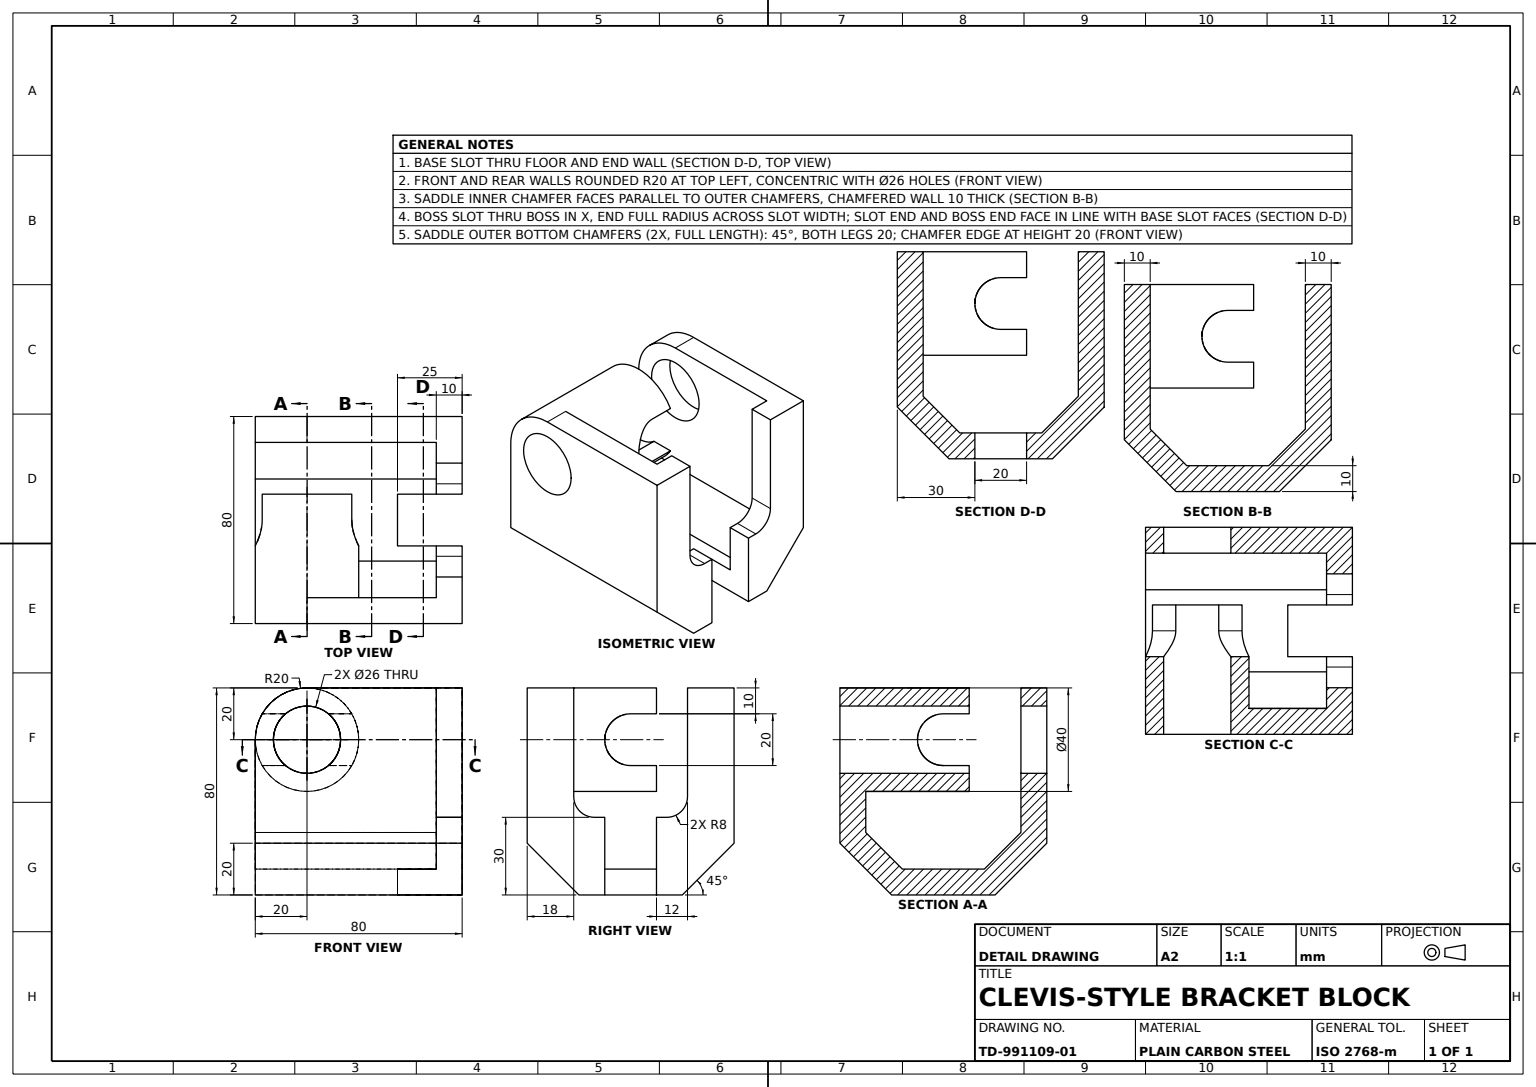
from build123d import *

# Parameters (mm, degrees)
SADDLE_BODY_DEPTH     = 40
ARM_TOP_ROUNDS_R20_R  = 20
SIDE_BOSS_DEPTH       = 10
BOSS_POCKET_SKETCH_W  = 20
BOSS_POCKET_SKETCH_H  = 10
BOSS_POCKET_CUT_DEPTH = 25
JOURNAL_BOSS_SKETCH_R = 20
JOURNAL_BOSS_DEPTH    = 40
BASE_SLOT_20X60_DEPTH = 98.979589711
JOURNAL_BORE_SKETCH_R = 13
JOURNAL_BORE_26_DEPTH = 121.0000001


with BuildPart() as part:
    # Saddle Profile Sketch → Saddle Body (new, symmetric)
    with BuildSketch(Plane(origin=(0, 0, 0), x_dir=(0, 0, -1), z_dir=(1, 0, 0))):
        Polygon((-20, 0), (20, 0), (40, 20), (40, 80), (30, 80), (30, 24.142135624), (15.857864376, 10), (-15.857864376, 10), (-30, 24.142135624), (-30, 80), (-40, 80), (-40, 20), align=None)
    extrude(amount=SADDLE_BODY_DEPTH, both=True)

    # Arm Top Rounds R20
    arm_top_rounds_r20_edges = [part.edges().sort_by_distance(p)[0] for p in [
        (-40, 80, 35),
        (-40, 80, -35),
    ]]
    fillet(arm_top_rounds_r20_edges, radius=ARM_TOP_ROUNDS_R20_R)

    # Side Boss Sketch → Side Boss (add)
    with BuildSketch(Plane(origin=(40, 0, 0), x_dir=(0, 0, -1), z_dir=(1, 0, 0))):
        with BuildLine():
            Line((-30, 80), (-22, 80))
            Line((-22, 80), (-22, 38))
            ThreePointArc((-22, 38), (-19.656854249, 32.343145751), (-14, 30))
            Line((-14, 30), (-10, 30))
            Line((-10, 30), (-10, 10))
            Line((-10, 10), (-15.857864376, 10))
            Line((-15.857864376, 10), (-30, 24.142135624))
            Line((-30, 24.142135624), (-30, 80))
        make_face()
        with BuildLine():
            Line((10, 30), (10, 10))
            Line((10, 10), (15.857864376, 10))
            Line((15.857864376, 10), (30, 24.142135624))
            Line((30, 24.142135624), (30, 80))
            Line((30, 80), (22, 80))
            Line((22, 80), (22, 38))
            ThreePointArc((22, 38), (19.656854249, 32.343145751), (14, 30))
            Line((14, 30), (10, 30))
        make_face()
    extrude(amount=-SIDE_BOSS_DEPTH)

    # Boss Pocket Sketch → Boss Pocket Cut (cut)
    with BuildSketch(Plane(origin=(40, 0, 0), x_dir=(0, 0, -1), z_dir=(1, 0, 0))):
        with Locations((0, 5)):
            Rectangle(BOSS_POCKET_SKETCH_W, BOSS_POCKET_SKETCH_H)
    extrude(amount=-BOSS_POCKET_CUT_DEPTH, mode=Mode.SUBTRACT)

    # Journal Boss Sketch → Journal Boss (add)
    with BuildSketch(Plane(origin=(0, 0, 30), x_dir=(-1, 0, 0), z_dir=(0, 0, -1))):
        with Locations(Location((20, 60, 0), (0, 0, 90))):
            Circle(JOURNAL_BOSS_SKETCH_R)
    extrude(amount=JOURNAL_BOSS_DEPTH)

    # Base Slot Sketch → Base Slot 20x60 (cut, through all)
    with BuildSketch(Plane(origin=(0, 0, 0), x_dir=(0, 0, -1), z_dir=(1, 0, 0))):
        with BuildLine():
            Line((0, 70), (14.531264235, 70))
            Line((14.531264235, 70), (14.531264235, 50))
            Line((14.531264235, 50), (0, 50))
            ThreePointArc((0, 50), (-10, 60), (0, 70))
        make_face()
    extrude(amount=-BASE_SLOT_20X60_DEPTH, mode=Mode.SUBTRACT)

    # Journal Bore Sketch → Journal Bore Ø26 (cut, through all)
    with BuildSketch(Plane(origin=(0, 0, -40), x_dir=(-1, 0, 0), z_dir=(0, 0, -1))):
        with Locations((20, 60)):
            Circle(JOURNAL_BORE_SKETCH_R)
    extrude(amount=-JOURNAL_BORE_26_DEPTH, mode=Mode.SUBTRACT)


solid = part.part
